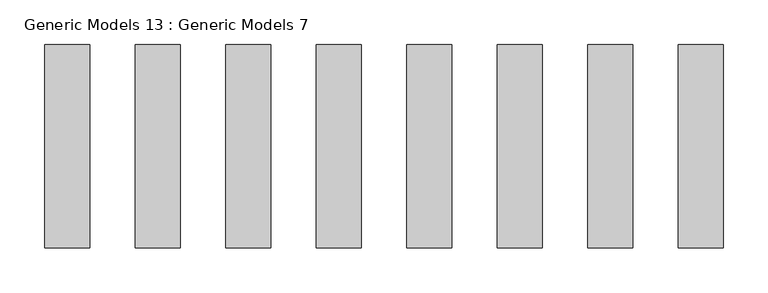
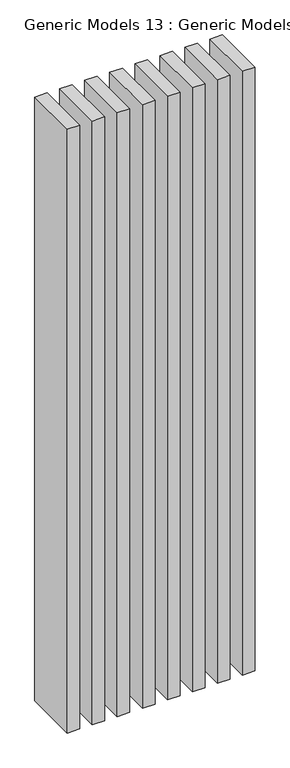
"""IFC4 building model written with IfcOpenShell, lengths in millimetres: proxy geometry, Generic Models 13 : Generic Models 7."""

from ifc_helpers import new_model, si_unit, frame, origin, place, context, project, spatial, polyline, outline, extrude, source, transform, mapped, element, save


def generic_models_13_generic_models_7_57cb182b(model_context):
    return source(origin(), model_context, "Body", "SweptSolid", [
        extrude(outline(polyline([(-9534.0519394, -11116.4679047), (-9584.8519394, -11116.4679047), (-9584.8519394, -10887.8679047), (-9534.0519394, -10887.8679047), (-9534.0519394, -11116.4679047)])), frame((0.0, 0.0, 6400.8), z_axis=(0.0, 0.0, 1.0), x_axis=(1.0, 0.0, 0.0)), (0.0, 0.0, 1.0), 2590.8),
        extrude(outline(polyline([(-9432.4519394, -11116.4679047), (-9483.2519394, -11116.4679047), (-9483.2519394, -10887.8679047), (-9432.4519394, -10887.8679047), (-9432.4519394, -11116.4679047)])), frame((0.0, 0.0, 6400.8), z_axis=(0.0, 0.0, 1.0), x_axis=(1.0, 0.0, 0.0)), (0.0, 0.0, 1.0), 2590.8),
        extrude(outline(polyline([(-9330.8519394, -11116.4679047), (-9381.6519394, -11116.4679047), (-9381.6519394, -10887.8679047), (-9330.8519394, -10887.8679047), (-9330.8519394, -11116.4679047)])), frame((0.0, 0.0, 6400.8), z_axis=(0.0, 0.0, 1.0), x_axis=(1.0, 0.0, 0.0)), (0.0, 0.0, 1.0), 2590.8),
        extrude(outline(polyline([(-9229.2519394, -11116.4679047), (-9280.0519394, -11116.4679047), (-9280.0519394, -10887.8679047), (-9229.2519394, -10887.8679047), (-9229.2519394, -11116.4679047)])), frame((0.0, 0.0, 6400.8), z_axis=(0.0, 0.0, 1.0), x_axis=(1.0, 0.0, 0.0)), (0.0, 0.0, 1.0), 2590.8),
        extrude(outline(polyline([(-9127.6519394, -11116.4679047), (-9178.4519394, -11116.4679047), (-9178.4519394, -10887.8679047), (-9127.6519394, -10887.8679047), (-9127.6519394, -11116.4679047)])), frame((0.0, 0.0, 6400.8), z_axis=(0.0, 0.0, 1.0), x_axis=(1.0, 0.0, 0.0)), (0.0, 0.0, 1.0), 2590.8),
        extrude(outline(polyline([(-9026.0519394, -11116.4679047), (-9076.8519394, -11116.4679047), (-9076.8519394, -10887.8679047), (-9026.0519394, -10887.8679047), (-9026.0519394, -11116.4679047)])), frame((0.0, 0.0, 6400.8), z_axis=(0.0, 0.0, 1.0), x_axis=(1.0, 0.0, 0.0)), (0.0, 0.0, 1.0), 2590.8),
        extrude(outline(polyline([(-8924.4519394, -11116.4679047), (-8975.2519394, -11116.4679047), (-8975.2519394, -10887.8679047), (-8924.4519394, -10887.8679047), (-8924.4519394, -11116.4679047)])), frame((0.0, 0.0, 6400.8), z_axis=(0.0, 0.0, 1.0), x_axis=(1.0, 0.0, 0.0)), (0.0, 0.0, 1.0), 2590.8),
        extrude(outline(polyline([(-8822.8519394, -11116.4679047), (-8873.6519394, -11116.4679047), (-8873.6519394, -10887.8679047), (-8822.8519394, -10887.8679047), (-8822.8519394, -11116.4679047)])), frame((0.0, 0.0, 6400.8), z_axis=(0.0, 0.0, 1.0), x_axis=(1.0, 0.0, 0.0)), (0.0, 0.0, 1.0), 2590.8),
    ])


if __name__ == "__main__":
    model = new_model("IFC4")
    model_context = context("Model", 3, world=origin())
    ifc_project = project(units=[si_unit("LENGTHUNIT", "METRE", prefix="MILLI")], contexts=[model_context])
    site = spatial("IfcSite", under=ifc_project)
    building = spatial("IfcBuilding", under=site)
    placement = place(None, origin())
    generic_models_13_generic_models_7_shape = generic_models_13_generic_models_7_57cb182b(model_context)
    element("IfcBuildingElementProxy", 1, Name="Generic Models 13 : Generic Models 7", ObjectType="Generic Models 13 : Generic Models 7", at=placement, inside=building, context=model_context, shape_type="MappedRepresentation", body=[
        mapped(generic_models_13_generic_models_7_shape, transform((0.0, 0.0, 0.0), x_axis=(1.0, 0.0, 0.0), y_axis=(0.0, 1.0, 0.0), z_axis=(0.0, 0.0, 1.0))),
    ])
    save(model, "model.ifc")

# Revit data of these elements
# Element 1 (IfcBuildingElementProxy, "Generic Models 13 : Generic Models 7")
#   Materials on its faces: "TEAK BROWN COLOUR"
# Materials
#   "TEAK BROWN COLOUR": class "Generic", colour RGB 120 120 120, transparency 0, Cost = 0
